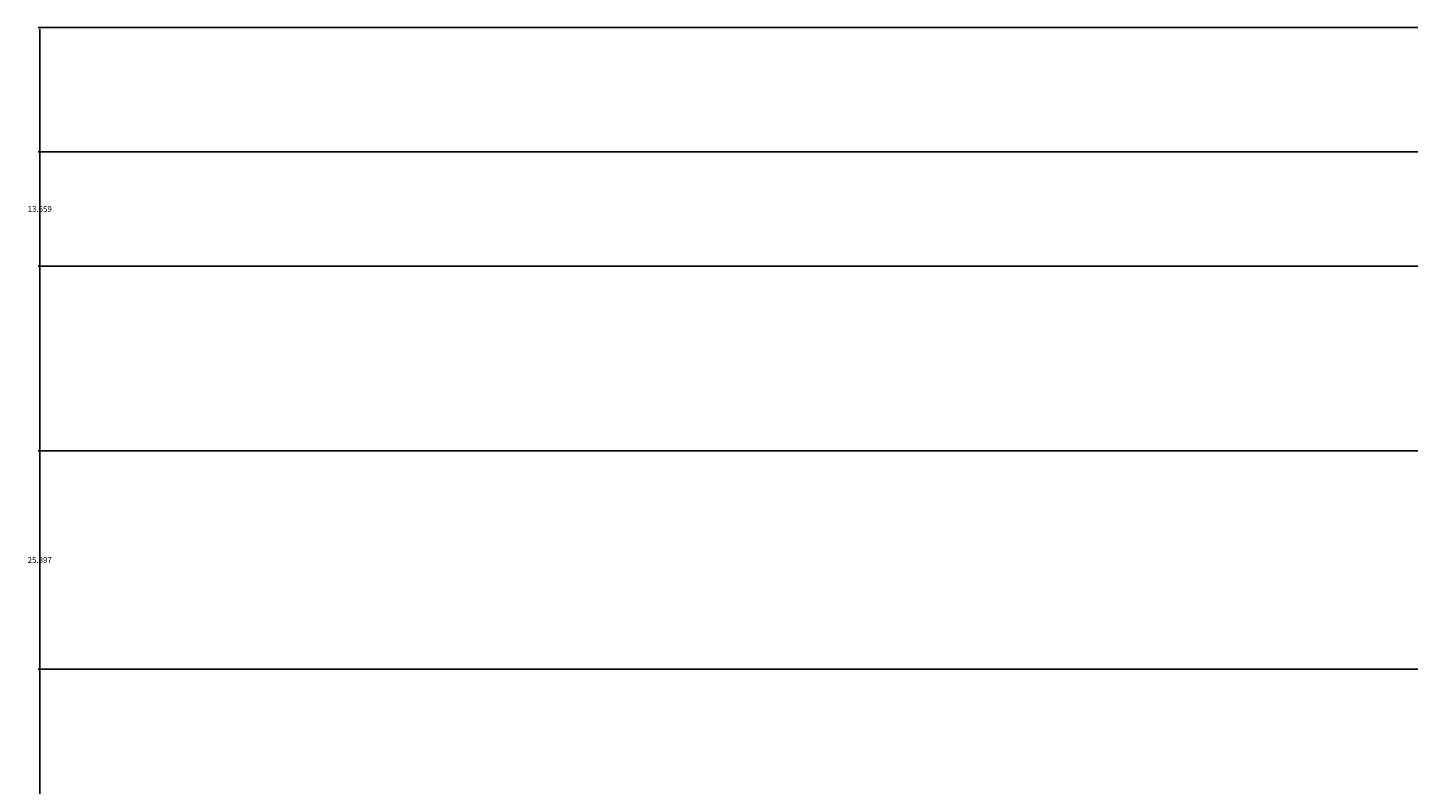
# Model space of a CAD drawing. Units: inches. Extents: x -145 to 510, y 5 to 386.
# Tile 9 of 25: x -145 to 18, y 266 to 356. Entities that reach past the tile are written whole.
import ezdxf

# ---------------------------------------------------------------- set-up
doc = ezdxf.new("R2010")
doc.units = ezdxf.units.IN
doc.header["$MEASUREMENT"] = 0
doc.layers.add('A-ANNO-DIMS', color=2, linetype='Continuous', lineweight=18)
doc.styles.get("Standard").update_dxf_attribs({"font": 'arial.ttf'})
doc.dimstyles.get("Standard").update_dxf_attribs({"dimtxt": 0.6875, "dimasz": 0.18, "dimexe": 0.18, "dimexo": 0.0625, "dimgap": 0.09, "dimtad": 0, "dimtih": 1, "dimtoh": 1, "dimdec": 4, "dimzin": 0, "dimdsep": 46, "dimlunit": 4, "dimtxsty": 'Standard', "dimcen": 0.09, "dimadec": 0, "dimazin": 0, "dimtfac": 1, "dimtdec": 4, "dimtofl": 0, "dimtmove": 0, "dimatfit": 3, "dimfxl": 1, "dimtolj": 1, "dimtzin": 0, "dimarcsym": 0})

# ---------------------------------------------------------------- blocks, each defined once
blk = doc.blocks.new('*D19')
at = {"layer": 'A-ANNO-DIMS', "color": 0, "lineweight": -2, "transparency": 16777216}
for p, q in [((478.76, 355.89), (-144.05, 355.89)), ((-143.87, 355.71), (-143.87, 218.33)), ((-143.87, 80.07), (-143.87, 217.45)), ((-114.04, 79.89), (-144.05, 79.89))]:
    blk.add_line(p, q, dxfattribs=at)
at = {"layer": 'A-ANNO-DIMS', "color": 0, "transparency": 16777216}
for points in [[(-143.9, 355.71), (-143.84, 355.71), (-143.87, 355.89)], [(-143.9, 80.07), (-143.84, 80.07), (-143.87, 79.89)]]:
    blk.add_solid(points, dxfattribs=at)
at = {"layer": 'Defpoints', "color": 0, "transparency": 16777216}
for p in [(-143.87, 355.89), (478.83, 355.89), (-113.97, 79.89)]:
    blk.add_point(p, dxfattribs=at)
at = {"layer": 'A-ANNO-DIMS', "color": 0, "transparency": 16777216, "insert": (-143.87, 217.89), "char_height": 0.688, "attachment_point": 5}
blk.add_mtext('\\A1;276', dxfattribs=at)
blk = doc.blocks.new('*D21')
at = {"layer": 'A-ANNO-DIMS', "color": 0, "lineweight": -2, "transparency": 16777216}
for p, q in [((34.21, 327.61), (-144.05, 327.61)), ((-143.87, 327.43), (-143.87, 264.19)), ((-143.87, 200.07), (-143.87, 263.31)), ((69.71, 199.89), (-144.05, 199.89))]:
    blk.add_line(p, q, dxfattribs=at)
at = {"layer": 'A-ANNO-DIMS', "color": 0, "transparency": 16777216}
for points in [[(-143.9, 327.43), (-143.84, 327.43), (-143.87, 327.61)], [(-143.9, 200.07), (-143.84, 200.07), (-143.87, 199.89)]]:
    blk.add_solid(points, dxfattribs=at)
at = {"layer": 'Defpoints', "color": 0, "transparency": 16777216}
for p in [(-143.87, 327.61), (34.27, 327.61), (69.78, 199.89)]:
    blk.add_point(p, dxfattribs=at)
at = {"layer": 'A-ANNO-DIMS', "color": 0, "transparency": 16777216, "insert": (-143.87, 263.75), "char_height": 0.688, "attachment_point": 5}
blk.add_mtext('\\A1;127.72', dxfattribs=at)
blk = doc.blocks.new('*D22')
at = {"layer": 'A-ANNO-DIMS', "color": 0, "lineweight": -2, "transparency": 16777216}
for p, q in [((34.21, 341.17), (-144.05, 341.17)), ((-143.87, 340.99), (-143.87, 334.83)), ((-143.87, 327.79), (-143.87, 333.95)), ((34.21, 327.61), (-144.05, 327.61))]:
    blk.add_line(p, q, dxfattribs=at)
at = {"layer": 'A-ANNO-DIMS', "color": 0, "transparency": 16777216}
for points in [[(-143.9, 340.99), (-143.84, 340.99), (-143.87, 341.17)], [(-143.9, 327.79), (-143.84, 327.79), (-143.87, 327.61)]]:
    blk.add_solid(points, dxfattribs=at)
at = {"layer": 'Defpoints', "color": 0, "transparency": 16777216}
for p in [(-143.87, 341.17), (34.27, 341.17), (34.27, 327.61)]:
    blk.add_point(p, dxfattribs=at)
at = {"layer": 'A-ANNO-DIMS', "color": 0, "transparency": 16777216, "insert": (-143.87, 334.39), "char_height": 0.688, "attachment_point": 5}
blk.add_mtext('\\A1;13.559', dxfattribs=at)
blk = doc.blocks.new('*D26')
at = {"layer": 'A-ANNO-DIMS', "color": 0, "lineweight": -2, "transparency": 16777216}
for p, q in [((95.08, 305.74), (-144.05, 305.74)), ((-143.87, 305.56), (-143.87, 253.26)), ((-143.87, 200.07), (-143.87, 252.38)), ((95.08, 199.89), (-144.05, 199.89))]:
    blk.add_line(p, q, dxfattribs=at)
at = {"layer": 'A-ANNO-DIMS', "color": 0, "transparency": 16777216}
for points in [[(-143.9, 305.56), (-143.84, 305.56), (-143.87, 305.74)], [(-143.9, 200.07), (-143.84, 200.07), (-143.87, 199.89)]]:
    blk.add_solid(points, dxfattribs=at)
at = {"layer": 'Defpoints', "color": 0, "transparency": 16777216}
for p in [(-143.87, 305.74), (95.14, 305.74), (95.14, 199.89)]:
    blk.add_point(p, dxfattribs=at)
at = {"layer": 'A-ANNO-DIMS', "color": 0, "transparency": 16777216, "insert": (-143.87, 252.82), "char_height": 0.688, "attachment_point": 5}
blk.add_mtext('\\A1;105.85', dxfattribs=at)
blk = doc.blocks.new('*D27')
at = {"layer": 'A-ANNO-DIMS', "color": 0, "lineweight": -2, "transparency": 16777216}
for p, q in [((244.23, 279.84), (-144.05, 279.84)), ((-143.87, 279.66), (-143.87, 240.31)), ((-143.87, 200.07), (-143.87, 239.43)), ((218.29, 199.89), (-144.05, 199.89))]:
    blk.add_line(p, q, dxfattribs=at)
at = {"layer": 'A-ANNO-DIMS', "color": 0, "transparency": 16777216}
for points in [[(-143.9, 279.66), (-143.84, 279.66), (-143.87, 279.84)], [(-143.9, 200.07), (-143.84, 200.07), (-143.87, 199.89)]]:
    blk.add_solid(points, dxfattribs=at)
at = {"layer": 'Defpoints', "color": 0, "transparency": 16777216}
for p in [(-143.87, 279.84), (244.29, 279.84), (218.36, 199.89)]:
    blk.add_point(p, dxfattribs=at)
at = {"layer": 'A-ANNO-DIMS', "color": 0, "transparency": 16777216, "insert": (-143.87, 239.87), "char_height": 0.688, "attachment_point": 5}
blk.add_mtext('\\A1;79.95', dxfattribs=at)
blk = doc.blocks.new('*D28')
at = {"layer": 'A-ANNO-DIMS', "color": 0, "lineweight": -2, "transparency": 16777216}
for p, q in [((244.23, 305.74), (-144.05, 305.74)), ((-143.87, 305.56), (-143.87, 293.23)), ((-143.87, 280.02), (-143.87, 292.35)), ((244.23, 279.84), (-144.05, 279.84))]:
    blk.add_line(p, q, dxfattribs=at)
at = {"layer": 'A-ANNO-DIMS', "color": 0, "transparency": 16777216}
for points in [[(-143.9, 305.56), (-143.84, 305.56), (-143.87, 305.74)], [(-143.9, 280.02), (-143.84, 280.02), (-143.87, 279.84)]]:
    blk.add_solid(points, dxfattribs=at)
at = {"layer": 'Defpoints', "color": 0, "transparency": 16777216}
for p in [(-143.87, 305.74), (244.29, 305.74), (244.29, 279.84)]:
    blk.add_point(p, dxfattribs=at)
at = {"layer": 'A-ANNO-DIMS', "color": 0, "transparency": 16777216, "insert": (-143.87, 292.79), "char_height": 0.688, "attachment_point": 5}
blk.add_mtext('\\A1;25.897', dxfattribs=at)

msp = doc.modelspace()

# ---------------------------------------------------------------- dimensions: what is measured, and where the dimension line sits
at = {"layer": 'A-ANNO-DIMS'}
for base, p1, p2, override, picture, middle in [((-143.8737, 355.8905), (-113.9737, 79.8905), (478.8263, 355.8905), {"dimdec": 0, "dimlfac": 1, "dimrnd": 0, "dimzin": 0, "dimdsep": 46, "dimlunit": 2}, '*D19', (-143.8737, 217.8905)), ((-143.8737, 341.168), (34.2706, 327.6093), (34.2706, 341.168), {"dimdec": 3, "dimlfac": 1, "dimrnd": 0, "dimzin": 0, "dimdsep": 46, "dimlunit": 2}, '*D22', (-143.8737, 334.3886)), ((-143.8737, 327.6093), (69.7763, 199.8905), (34.2706, 327.6093), {"dimdec": 2, "dimlfac": 1, "dimrnd": 0, "dimzin": 0, "dimdsep": 46, "dimlunit": 2}, '*D21', (-143.8737, 263.7499)), ((-143.8737, 305.7416), (95.1414, 199.8905), (95.1414, 305.7416), {"dimdec": 2, "dimlfac": 1, "dimrnd": 0, "dimzin": 0, "dimdsep": 46, "dimlunit": 2}, '*D26', (-143.8737, 252.8161)), ((-143.8737, 305.7416), (244.2916, 279.8443), (244.2916, 305.7416), {"dimdec": 3, "dimlfac": 1, "dimrnd": 0, "dimzin": 0, "dimdsep": 46, "dimlunit": 2}, '*D28', (-143.8737, 292.793)), ((-143.8737, 279.8443), (218.3571, 199.8905), (244.2916, 279.8443), {"dimdec": 2, "dimlfac": 1, "dimrnd": 0, "dimzin": 0, "dimdsep": 46, "dimlunit": 2}, '*D27', (-143.8737, 239.8674))]:
    dim = msp.add_linear_dim(base=base, p1=p1, p2=p2, angle=90, dimstyle='Standard', override=override, dxfattribs=at)
    dim.commit()
    dim.dimension.update_dxf_attribs({"geometry": picture, "text_midpoint": middle})

doc.saveas('drawing.dxf')
